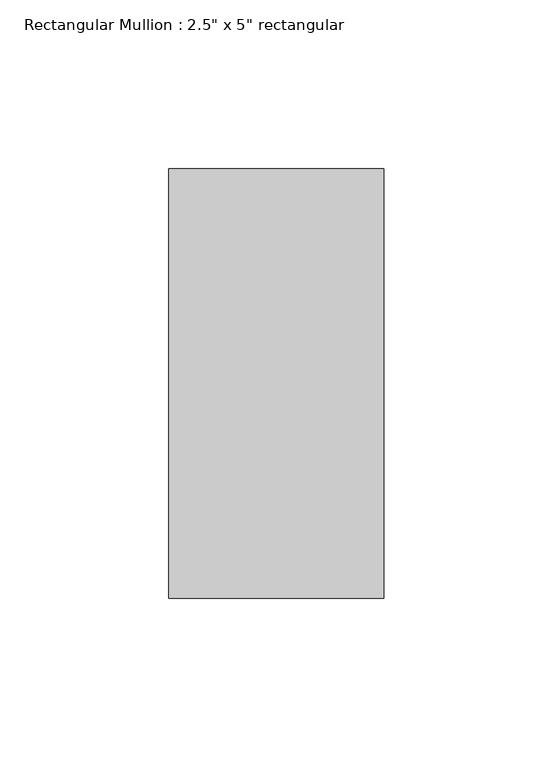
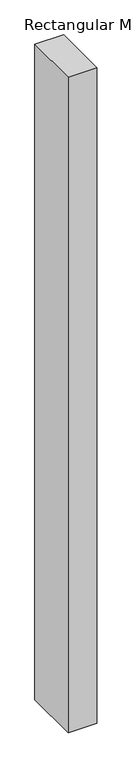
"""IFC4 building model written with IfcOpenShell, lengths in millimetres: member geometry."""

from ifc_helpers import new_model, si_unit, frame, origin, place, context, project, spatial, polyline, outline, extrude, source, transform, mapped, element, save


def member_2f32d0be(model_context):
    return source(origin(), model_context, "Body", "SweptSolid", [
        extrude(outline(polyline([(0.0, 63.5), (0.0, -63.5), (-63.5, -63.5), (-63.5, 63.5), (0.0, 63.5)])), frame((0.0, 0.0, -1533.754744), z_axis=(0.0, 0.0, 1.0), x_axis=(1.0, 0.0, 0.0)), (0.0, 0.0, 1.0), 1533.754744),
    ])


if __name__ == "__main__":
    model = new_model("IFC4")
    model_context = context("Model", 3, world=origin())
    ifc_project = project(units=[si_unit("LENGTHUNIT", "METRE", prefix="MILLI")], contexts=[model_context])
    site = spatial("IfcSite", under=ifc_project)
    building = spatial("IfcBuilding", under=site)
    placement = place(None, origin())
    member_shape = member_2f32d0be(model_context)
    element("IfcMember", 1, ObjectType="Rectangular Mullion : 2.5\" x 5\" rectangular", at=placement, inside=building, context=model_context, shape_type="MappedRepresentation", body=[
        mapped(member_shape, transform((0.0, 0.0, 0.0), x_axis=(1.0, 0.0, 0.0), y_axis=(0.0, 1.0, 0.0), z_axis=(0.0, 0.0, 1.0))),
    ])
    save(model, "model.ifc")

# Revit data of these elements
# Type "Rectangular Mullion : 2.5\" x 5\" rectangular"
#   built-in parameter 1007304 = 0.416667 (stored number, unit not read)
#   built-in parameter 1007301 = 0.104167 (stored number, unit not read)
#   built-in parameter 1007300 = 0.104167 (stored number, unit not read)
# Element 1 (IfcMember, "Rectangular Mullion : 2.5\" x 5\" rectangular")
#   Materials on its faces: "Aluminum"
# Materials
#   "Aluminum": class "Metal", colour RGB 247 247 247, transparency 0, Description = "Aluminum 6061", Cost = 0
